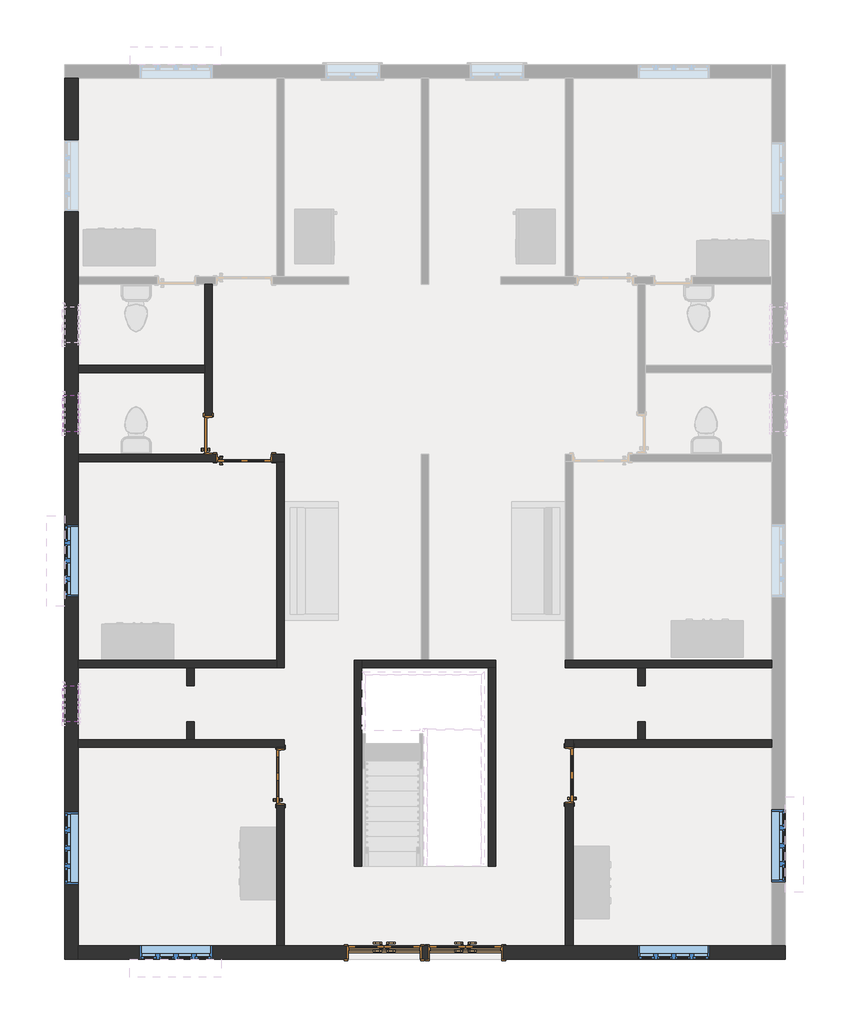
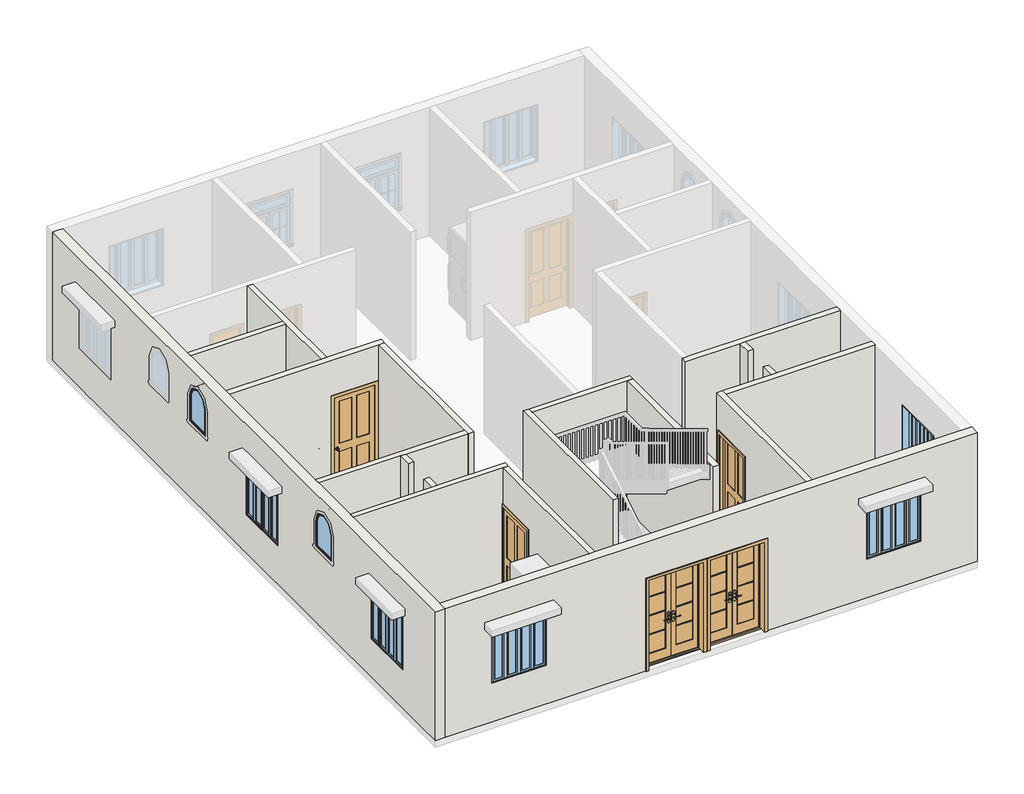
# One storey, part 1 of 4: 19 walls, 7 windows, 6 doors.
"""IFC4 building model written with IfcOpenShell, lengths in millimetres."""

from ifc_helpers import new_model, si_unit, frame, origin, origin_with_axes, place, context, project, spatial, polyline, circle_curve, outline, extrude, faceted_brep, transform, mapped, element, save
from ifc_brep_helpers import plane_surface, revolved_surface, advanced_brep
from components import door_exterior_double_full_glass_wood_clad_exterior_door_4_x_3788f36b, door_a823658d, door_68a706ac, door_3f5f64ee, window_casement_multi_sash_horizontal_main_windows_4_x_7_0e27d311, window_casement_multi_sash_horizontal_main_windows_4_x_7_c0e1ebbb, window_2fd4accf

model = new_model("IFC4")

# Units and contexts
model_context = context("Model", 3, world=origin())
ifc_project = project(units=[si_unit("LENGTHUNIT", "METRE", prefix="MILLI")], contexts=[model_context])

# Site, building, storey
site = spatial("IfcSite", under=ifc_project)
building = spatial("IfcBuilding", under=site)
storey = spatial("IfcBuildingStorey", under=building, Elevation=0.0)

# Doors
placement = place(None, origin())
door_exterior_double_full_glass_wood_clad_exterior_door_4_x_shape = door_exterior_double_full_glass_wood_clad_exterior_door_4_x_3788f36b(model_context)
element("IfcDoor", 1, ObjectType="Door-Exterior-Double-Full Glass-Wood_Clad : EXTERIOR DOOR 4' X 7'", at=placement, inside=storey, context=model_context, shape_type="MappedRepresentation", body=[
    mapped(door_exterior_double_full_glass_wood_clad_exterior_door_4_x_shape, transform((-10224.7771954, -6414.7977897, 0.0), x_axis=(1.0, 0.0, 0.0), y_axis=(0.0, 1.0, 0.0), z_axis=(0.0, 0.0, 1.0))),
])
element("IfcDoor", 2, ObjectType="Door-Exterior-Double-Full Glass-Wood_Clad : EXTERIOR DOOR 4' X 7'", at=placement, inside=storey, context=model_context, shape_type="MappedRepresentation", body=[
    mapped(door_exterior_double_full_glass_wood_clad_exterior_door_4_x_shape, transform((-8853.1771954, -6414.7977897, 0.0), x_axis=(1.0, 0.0, 0.0), y_axis=(0.0, 1.0, 0.0), z_axis=(0.0, 0.0, 1.0))),
])
door_shape = door_a823658d(model_context)
element("IfcDoor", 3, ObjectType="Door-Interior-Single-4_Panel-Wood : 36\" x 84\"", at=placement, inside=storey, context=model_context, shape_type="MappedRepresentation", body=[
    mapped(door_shape, transform((-7097.4021954, -3420.7727897, 0.0), x_axis=(0.0, 1.0, 0.0), y_axis=(-1.0, 0.0, 0.0), z_axis=(0.0, 0.0, 1.0))),
])
element("IfcDoor", 4, ObjectType="Door-Interior-Single-4_Panel-Wood : 36\" x 84\"", at=placement, inside=storey, context=model_context, shape_type="MappedRepresentation", body=[
    mapped(door_shape, transform((-12586.9771954, 1935.9816069, 0.0), x_axis=(1.0, 0.0, 0.0), y_axis=(0.0, 1.0, 0.0), z_axis=(0.0, 0.0, 1.0))),
])
door_2_shape = door_68a706ac(model_context)
element("IfcDoor", 5, ObjectType="Door-Interior-Single-4_Panel-Wood : 36\" x 84\"", at=placement, inside=storey, context=model_context, shape_type="MappedRepresentation", body=[
    mapped(door_2_shape, transform((-11980.5521954, -3446.1727897, 0.0), x_axis=(0.0, 1.0, 0.0), y_axis=(-1.0, 0.0, 0.0), z_axis=(0.0, 0.0, 1.0))),
])
door_3_shape = door_3f5f64ee(model_context)
element("IfcDoor", 6, ObjectType="Door-Interior-Single-Flush_Panel-Wood : 24\" x 84\"", at=placement, inside=storey, context=model_context, shape_type="MappedRepresentation", body=[
    mapped(door_3_shape, transform((-13199.7521954, 2320.1566069, 0.0), x_axis=(0.0, 1.0, 0.0), y_axis=(-1.0, 0.0, 0.0), z_axis=(0.0, 0.0, 1.0))),
])

# Walls
element("IfcWall", 7, ObjectType="INNER WALL 5\"", at=placement, inside=storey, context=model_context, shape_type="SweptSolid", body=[
    extrude(outline(polyline([(-13260.0771954, 3373.7272103), (-15395.2646954, 3373.7272103), (-15395.2646954, 3500.7272103), (-13260.0771954, 3500.7272103), (-13260.0771954, 3373.7272103)])), origin_with_axes(), (0.0, 0.0, 1.0), 3048.0),
])
element("IfcWall", 8, ObjectType="INNER WALL 5\"", at=placement, inside=storey, context=model_context, shape_type="Brep", body=[
    faceted_brep([(-13260.0771954, 4872.3272103, 3048.0), (-13260.0771954, 4872.3272103, 0.0), (-13260.0771954, 3500.7272103, 0.0), (-13260.0771954, 3373.7272103, 0.0), (-13260.0771954, 2650.3566069, 0.0), (-13260.0771954, 2650.3566069, 2159.0), (-13260.0771954, 2002.6566069, 2159.0), (-13260.0771954, 2002.6566069, 3048.0), (-13260.0771954, 3373.7272103, 3048.0), (-13260.0771954, 3500.7272103, 3048.0), (-13133.0771954, 4872.3272103, 0.0), (-13133.0771954, 4872.3272103, 3048.0), (-13133.0771954, 2002.6566069, 3048.0), (-13133.0771954, 2002.6566069, 2159.0), (-13133.0771954, 2650.3566069, 2159.0), (-13133.0771954, 2650.3566069, 0.0)], [[[0, 1, 2, 3, 4, 5, 6, 7, 8, 9]], [[10, 11, 12, 13, 14, 15]], [[1, 10, 15, 4, 3, 2]], [[1, 0, 11, 10]], [[12, 7, 6, 13]], [[14, 5, 4, 15]], [[5, 14, 13, 6]], [[0, 9, 8, 7, 12, 11]]]),
])
element("IfcWall", 9, ObjectType="INNER WALL 5\"", at=placement, inside=storey, context=model_context, shape_type="Brep", body=[
    faceted_brep([(-15395.2646954, 1875.6566069, 3048.0), (-15395.2646954, 1875.6566069, 0.0), (-13069.5771954, 1875.6566069, 0.0), (-13069.5771954, 1875.6566069, 2159.0), (-12104.3771954, 1875.6566069, 2159.0), (-12104.3771954, 1875.6566069, 0.0), (-12040.8771954, 1875.6566069, 0.0), (-11913.8771954, 1875.6566069, 0.0), (-11913.8771954, 1875.6566069, 3048.0), (-12040.8771954, 1875.6566069, 3048.0), (-15395.2646954, 2002.6566069, 0.0), (-15395.2646954, 2002.6566069, 3048.0), (-13260.0771954, 2002.6566069, 3048.0), (-13133.0771954, 2002.6566069, 3048.0), (-11913.8771954, 2002.6566069, 3048.0), (-11913.8771954, 2002.6566069, 0.0), (-12104.3771954, 2002.6566069, 0.0), (-12104.3771954, 2002.6566069, 2159.0), (-13069.5771954, 2002.6566069, 2159.0), (-13069.5771954, 2002.6566069, 0.0), (-13133.0771954, 2002.6566069, 0.0), (-13133.0771954, 2002.6566069, 2159.0), (-13260.0771954, 2002.6566069, 2159.0), (-13260.0771954, 2002.6566069, 0.0), (-13260.0771954, 1989.9566069, 0.0), (-13133.0771954, 1989.9566069, 0.0), (-13133.0771954, 1989.9566069, 2159.0), (-13260.0771954, 1989.9566069, 2159.0)], [[[0, 1, 2, 3, 4, 5, 6, 7, 8, 9]], [[10, 11, 12, 13, 14, 15, 16, 17, 18, 19, 20, 21, 22, 23]], [[1, 10, 23, 24, 25, 20, 19, 2]], [[15, 7, 6, 5, 16]], [[1, 0, 11, 10]], [[8, 7, 15, 14]], [[4, 17, 16, 5]], [[17, 4, 3, 18]], [[18, 3, 2, 19]], [[25, 26, 21, 20]], [[27, 24, 23, 22]], [[26, 27, 22, 21]], [[26, 25, 24, 27]], [[0, 9, 8, 14, 13, 12, 11]]]),
])
element("IfcWall", 10, ObjectType="INNER WALL 5\"", at=placement, inside=storey, context=model_context, shape_type="Brep", body=[
    faceted_brep([(-12040.8771954, 1875.6566069, 0.0), (-12040.8771954, -1477.6727897, 0.0), (-12040.8771954, -1604.6727897, 0.0), (-12040.8771954, -1604.6727897, 3048.0), (-12040.8771954, -1477.6727897, 3048.0), (-12040.8771954, 1875.6566069, 3048.0), (-11913.8771954, 1875.6566069, 0.0), (-11913.8771954, 1875.6566069, 3048.0), (-11913.8771954, -1604.6727897, 3048.0), (-11913.8771954, -1604.6727897, 0.0)], [[[0, 1, 2, 3, 4, 5]], [[6, 7, 8, 9]], [[2, 1, 0, 6, 9]], [[0, 5, 7, 6]], [[3, 2, 9, 8]], [[5, 4, 3, 8, 7]]]),
])
element("IfcWall", 11, ObjectType="INNER WALL 5\"", at=placement, inside=storey, context=model_context, shape_type="Brep", body=[
    faceted_brep([(-12040.8771954, -1477.6727897, 0.0), (-15395.2646954, -1477.6727897, 0.0), (-15395.2646954, -1477.6727897, 3048.0), (-12040.8771954, -1477.6727897, 3048.0), (-12040.8771954, -1604.6727897, 0.0), (-12040.8771954, -1604.6727897, 3048.0), (-13437.8771954, -1604.6727897, 3048.0), (-13564.8771954, -1604.6727897, 3048.0), (-15395.2646954, -1604.6727897, 3048.0), (-15395.2646954, -1604.6727897, 0.0), (-13564.8771954, -1604.6727897, 0.0), (-13437.8771954, -1604.6727897, 0.0)], [[[0, 1, 2, 3]], [[4, 5, 6, 7, 8, 9, 10, 11]], [[1, 0, 4, 11, 10, 9]], [[0, 3, 5, 4]], [[2, 1, 9, 8]], [[3, 2, 8, 7, 6, 5]]]),
])
element("IfcWall", 12, ObjectType="INNER WALL 5\"", at=placement, inside=storey, context=model_context, shape_type="Brep", body=[
    faceted_brep([(-15395.2646954, -2950.8727897, 0.0), (-12040.8771954, -2950.8727897, 0.0), (-11913.8771954, -2950.8727897, 0.0), (-11913.8771954, -2950.8727897, 3048.0), (-12040.8771954, -2950.8727897, 3048.0), (-15395.2646954, -2950.8727897, 3048.0), (-15395.2646954, -2823.8727897, 0.0), (-15395.2646954, -2823.8727897, 3048.0), (-13564.8771954, -2823.8727897, 3048.0), (-13437.8771954, -2823.8727897, 3048.0), (-11913.8771954, -2823.8727897, 3048.0), (-11913.8771954, -2823.8727897, 0.0), (-13437.8771954, -2823.8727897, 0.0), (-13564.8771954, -2823.8727897, 0.0)], [[[0, 1, 2, 3, 4, 5]], [[6, 7, 8, 9, 10, 11, 12, 13]], [[2, 1, 0, 6, 13, 12, 11]], [[0, 5, 7, 6]], [[3, 2, 11, 10]], [[5, 4, 3, 10, 9, 8, 7]]]),
])
element("IfcWall", 13, ObjectType="INNER WALL 5\"", at=placement, inside=storey, context=model_context, shape_type="SweptSolid", body=[
    extrude(outline(polyline([(-2950.8727897, 3048.0), (-2950.8727897, 0.0), (-2963.5727897, 0.0), (-2963.5727897, 2159.0), (-3928.7727897, 2159.0), (-3928.7727897, 0.0), (-6303.6727897, 0.0), (-6303.6727897, 3048.0), (-2950.8727897, 3048.0)])), frame((-12040.8771954, 0.0, 0.0), z_axis=(1.0, 0.0, 0.0), x_axis=(0.0, 1.0, 0.0)), (0.0, 0.0, 1.0), 127.0),
])
element("IfcWall", 14, ObjectType="INNER WALL 5\"", at=placement, inside=storey, context=model_context, shape_type="Brep", body=[
    faceted_brep([(-7037.0771954, -6303.6727897, 3048.0), (-7037.0771954, -6303.6727897, 0.0), (-7037.0771954, -3903.3727897, 0.0), (-7037.0771954, -3903.3727897, 2159.0), (-7037.0771954, -2938.1727897, 2159.0), (-7037.0771954, -2938.1727897, 0.0), (-7037.0771954, -2823.8727897, 0.0), (-7037.0771954, -2823.8727897, 3048.0), (-7037.0771954, -2950.8727897, 3048.0), (-7164.0771954, -6303.6727897, 0.0), (-7164.0771954, -6303.6727897, 3048.0), (-7164.0771954, -2823.8727897, 3048.0), (-7164.0771954, -2823.8727897, 0.0), (-7164.0771954, -2938.1727897, 0.0), (-7164.0771954, -2938.1727897, 2159.0), (-7164.0771954, -3903.3727897, 2159.0), (-7164.0771954, -3903.3727897, 0.0)], [[[0, 1, 2, 3, 4, 5, 6, 7, 8]], [[9, 10, 11, 12, 13, 14, 15, 16]], [[1, 9, 16, 2]], [[12, 6, 5, 13]], [[1, 0, 10, 9]], [[7, 6, 12, 11]], [[4, 14, 13, 5]], [[14, 4, 3, 15]], [[15, 3, 2, 16]], [[0, 8, 7, 11, 10]]]),
])
element("IfcWall", 15, ObjectType="INNER WALL 5\"", at=placement, inside=storey, context=model_context, shape_type="Brep", body=[
    faceted_brep([(-3684.2771954, -2823.8727897, 0.0), (-5817.8771954, -2823.8727897, 0.0), (-5944.8771954, -2823.8727897, 0.0), (-7037.0771954, -2823.8727897, 0.0), (-7037.0771954, -2823.8727897, 3048.0), (-5944.8771954, -2823.8727897, 3048.0), (-5817.8771954, -2823.8727897, 3048.0), (-3684.2771954, -2823.8727897, 3048.0), (-3684.2771954, -2950.8727897, 0.0), (-3684.2771954, -2950.8727897, 3048.0), (-7037.0771954, -2950.8727897, 3048.0), (-7037.0771954, -2950.8727897, 0.0)], [[[0, 1, 2, 3, 4, 5, 6, 7]], [[8, 9, 10, 11]], [[3, 2, 1, 0, 8, 11]], [[4, 3, 11, 10]], [[0, 7, 9, 8]], [[7, 6, 5, 4, 10, 9]]]),
])
element("IfcWall", 16, ObjectType="INNER WALL 5\"", at=placement, inside=storey, context=model_context, shape_type="Brep", body=[
    faceted_brep([(-3684.2771954, -1477.6727897, 0.0), (-7037.0771954, -1477.6727897, 0.0), (-7164.0771954, -1477.6727897, 0.0), (-7164.0771954, -1477.6727897, 3048.0), (-7037.0771954, -1477.6727897, 3048.0), (-3684.2771954, -1477.6727897, 3048.0), (-3684.2771954, -1604.6727897, 0.0), (-3684.2771954, -1604.6727897, 3048.0), (-5817.8771954, -1604.6727897, 3048.0), (-5944.8771954, -1604.6727897, 3048.0), (-7164.0771954, -1604.6727897, 3048.0), (-7164.0771954, -1604.6727897, 0.0), (-5944.8771954, -1604.6727897, 0.0), (-5817.8771954, -1604.6727897, 0.0)], [[[0, 1, 2, 3, 4, 5]], [[6, 7, 8, 9, 10, 11, 12, 13]], [[2, 1, 0, 6, 13, 12, 11]], [[0, 5, 7, 6]], [[3, 2, 11, 10]], [[5, 4, 3, 10, 9, 8, 7]]]),
])
element("IfcWall", 17, ObjectType="INNER WALL 5\"", at=placement, inside=storey, context=model_context, shape_type="SweptSolid", body=[
    extrude(outline(polyline([(-13564.8771954, -1909.4727897), (-13564.8771954, -1604.6727897), (-13437.8771954, -1604.6727897), (-13437.8771954, -1909.4727897), (-13564.8771954, -1909.4727897)])), origin_with_axes(), (0.0, 0.0, 1.0), 3048.0),
])
element("IfcWall", 18, ObjectType="INNER WALL 5\"", at=placement, inside=storey, context=model_context, shape_type="SweptSolid", body=[
    extrude(outline(polyline([(-13437.8771954, -2519.0727897), (-13437.8771954, -2823.8727897), (-13564.8771954, -2823.8727897), (-13564.8771954, -2519.0727897), (-13437.8771954, -2519.0727897)])), origin_with_axes(), (0.0, 0.0, 1.0), 3048.0),
])
element("IfcWall", 19, ObjectType="INNER WALL 5\"", at=placement, inside=storey, context=model_context, shape_type="SweptSolid", body=[
    extrude(outline(polyline([(-5817.8771954, -2519.0727897), (-5817.8771954, -2823.8727897), (-5944.8771954, -2823.8727897), (-5944.8771954, -2519.0727897), (-5817.8771954, -2519.0727897)])), origin_with_axes(), (0.0, 0.0, 1.0), 3048.0),
])
element("IfcWall", 20, ObjectType="INNER WALL 5\"", at=placement, inside=storey, context=model_context, shape_type="SweptSolid", body=[
    extrude(outline(polyline([(-5944.8771954, -1909.4727897), (-5944.8771954, -1604.6727897), (-5817.8771954, -1604.6727897), (-5817.8771954, -1909.4727897), (-5944.8771954, -1909.4727897)])), origin_with_axes(), (0.0, 0.0, 1.0), 3048.0),
])
element("IfcWall", 21, ObjectType="INNER WALL 5\"", at=placement, inside=storey, context=model_context, shape_type="Brep", body=[
    faceted_brep([(-10605.7771954, -4957.4727897, 0.0), (-10605.7771954, -1604.6727897, 0.0), (-10605.7771954, -1477.6727897, 0.0), (-10605.7771954, -1477.6727897, 3048.0), (-10605.7771954, -1604.6727897, 3048.0), (-10605.7771954, -4957.4727897, 3048.0), (-10732.7771954, -4957.4727897, 0.0), (-10732.7771954, -4957.4727897, 3048.0), (-10732.7771954, -1477.6727897, 3048.0), (-10732.7771954, -1477.6727897, 0.0)], [[[0, 1, 2, 3, 4, 5]], [[6, 7, 8, 9]], [[2, 1, 0, 6, 9]], [[0, 5, 7, 6]], [[3, 2, 9, 8]], [[5, 4, 3, 8, 7]]]),
])
element("IfcWall", 22, ObjectType="INNER WALL 5\"", at=placement, inside=storey, context=model_context, shape_type="Brep", body=[
    faceted_brep([(-10605.7771954, -1604.6727897, 0.0), (-8472.1771954, -1604.6727897, 0.0), (-8345.1771954, -1604.6727897, 0.0), (-8345.1771954, -1604.6727897, 3048.0), (-8472.1771954, -1604.6727897, 3048.0), (-10605.7771954, -1604.6727897, 3048.0), (-10605.7771954, -1477.6727897, 0.0), (-10605.7771954, -1477.6727897, 3048.0), (-9602.4771954, -1477.6727897, 3048.0), (-9475.4771954, -1477.6727897, 3048.0), (-8345.1771954, -1477.6727897, 3048.0), (-8345.1771954, -1477.6727897, 0.0), (-9475.4771954, -1477.6727897, 0.0), (-9602.4771954, -1477.6727897, 0.0)], [[[0, 1, 2, 3, 4, 5]], [[6, 7, 8, 9, 10, 11, 12, 13]], [[2, 1, 0, 6, 13, 12, 11]], [[0, 5, 7, 6]], [[3, 2, 11, 10]], [[5, 4, 3, 10, 9, 8, 7]]]),
])
element("IfcWall", 23, ObjectType="INNER WALL 5\"", at=placement, inside=storey, context=model_context, shape_type="SweptSolid", body=[
    extrude(outline(polyline([(-8472.1771954, -4957.4727897), (-8472.1771954, -1604.6727897), (-8345.1771954, -1604.6727897), (-8345.1771954, -4957.4727897), (-8472.1771954, -4957.4727897)])), origin_with_axes(), (0.0, 0.0, 1.0), 3048.0),
])
element("IfcWall", 24, ObjectType="OUTER WALL 9\"", at=placement, inside=storey, context=model_context, shape_type="AdvancedBrep", body=[
    advanced_brep(
    [(-15395.2646954, -6532.2727897, 0.0), (-15395.2646954, -6303.6727897, 0.0), (-15395.2646954, -2950.8727897, 0.0), (-15395.2646954, -2823.8727897, 0.0), (-15395.2646954, -1604.6727897, 0.0), (-15395.2646954, -1477.6727897, 0.0), (-15395.2646954, 1875.6566069, 0.0), (-15395.2646954, 2002.6566069, 0.0), (-15395.2646954, 3373.7272103, 0.0), (-15395.2646954, 3500.7272103, 0.0), (-15395.2646954, 4872.3272103, 0.0), (-15395.2646954, 4999.3272103, 0.0), (-15395.2646954, 8352.1272103, 0.0), (-15395.2646954, 8352.1272103, 3048.0), (-15395.2646954, 4999.3272103, 3048.0), (-15395.2646954, 4872.3272103, 3048.0), (-15395.2646954, 3500.7272103, 3048.0), (-15395.2646954, 3373.7272103, 3048.0), (-15395.2646954, 2002.6566069, 3048.0), (-15395.2646954, 1875.6566069, 3048.0), (-15395.2646954, -1477.6727897, 3048.0), (-15395.2646954, -1604.6727897, 3048.0), (-15395.2646954, -2823.8727897, 3048.0), (-15395.2646954, -2950.8727897, 3048.0), (-15395.2646954, -6303.6727897, 3048.0), (-15395.2646954, -6532.2727897, 3048.0), (-15395.2646954, -4043.0727897, 2260.6), (-15395.2646954, -4043.0727897, 914.4), (-15395.2646954, -5262.2727897, 914.4), (-15395.2646954, -5262.2727897, 2260.6), (-15395.2646954, 808.5919086, 2260.6), (-15395.2646954, 808.5919086, 914.4), (-15395.2646954, -410.6080914, 914.4), (-15395.2646954, -410.6080914, 2260.6), (-15395.2646954, 7310.7272103, 2260.6), (-15395.2646954, 7310.7272103, 914.4), (-15395.2646954, 6091.5272103, 914.4), (-15395.2646954, 6091.5272103, 2260.6), (-15395.2646954, -2519.0727897, 1828.8), (-15395.2646954, -2519.0727897, 2438.4), (-15395.2646954, -1909.4727897, 2438.4), (-15395.2646954, -1909.4727897, 1828.8), (-15395.2646954, 2383.3919086, 1828.8), (-15395.2646954, 2383.3919086, 2438.4), (-15395.2646954, 2992.9919086, 2438.4), (-15395.2646954, 2992.9919086, 1828.8), (-15395.2646954, 3881.7272103, 1828.8), (-15395.2646954, 3881.7272103, 2438.4), (-15395.2646954, 4491.3272103, 2438.4), (-15395.2646954, 4491.3272103, 1828.8), (-15623.8646954, -6532.2727897, 0.0), (-15623.8646954, -6532.2727897, 3048.0), (-15623.8646954, 8352.1272103, 3048.0), (-15623.8646954, 8352.1272103, 0.0), (-15623.8646954, -4043.0727897, 2260.6), (-15623.8646954, -5262.2727897, 2260.6), (-15623.8646954, -5262.2727897, 914.4), (-15623.8646954, -4043.0727897, 914.4), (-15623.8646954, 808.5919086, 2260.6), (-15623.8646954, -410.6080914, 2260.6), (-15623.8646954, -410.6080914, 914.4), (-15623.8646954, 808.5919086, 914.4), (-15623.8646954, 7310.7272103, 2260.6), (-15623.8646954, 6091.5272103, 2260.6), (-15623.8646954, 6091.5272103, 914.4), (-15623.8646954, 7310.7272103, 914.4), (-15623.8646954, -2519.0727897, 1828.8), (-15623.8646954, -1909.4727897, 1828.8), (-15623.8646954, -1909.4727897, 2438.4), (-15623.8646954, -2519.0727897, 2438.4), (-15623.8646954, 2383.3919086, 1828.8), (-15623.8646954, 2992.9919086, 1828.8), (-15623.8646954, 2992.9919086, 2438.4), (-15623.8646954, 2383.3919086, 2438.4), (-15623.8646954, 3881.7272103, 1828.8), (-15623.8646954, 4491.3272103, 1828.8), (-15623.8646954, 4491.3272103, 2438.4), (-15623.8646954, 3881.7272103, 2438.4)],
    [
        (0, 1),
        (1, 2),
        (2, 3),
        (3, 4),
        (4, 5),
        (5, 6),
        (6, 7),
        (7, 8),
        (8, 9),
        (9, 10),
        (10, 11),
        (11, 12),
        (12, 13),
        (13, 14),
        (14, 15),
        (15, 16),
        (16, 17),
        (17, 18),
        (18, 19),
        (19, 20),
        (20, 21),
        (21, 22),
        (22, 23),
        (23, 24),
        (24, 25),
        (25, 0),
        (26, 27),
        (27, 28),
        (28, 29),
        (29, 26),
        (30, 31),
        (31, 32),
        (32, 33),
        (33, 30),
        (34, 35),
        (35, 36),
        (36, 37),
        (37, 34),
        (38, 39),
        (39, 40, circle_curve(frame((-15395.2646954, -2214.2727897, 2438.4), z_axis=(-1.0, 0.0, 0.0), x_axis=(0.0, 1.0, 0.0)), 304.8)),
        (40, 41),
        (41, 38),
        (42, 43),
        (43, 44, circle_curve(frame((-15395.2646954, 2688.1919086, 2438.4), z_axis=(-1.0, 0.0, 0.0), x_axis=(0.0, 1.0, 0.0)), 304.8)),
        (44, 45),
        (45, 42),
        (46, 47),
        (47, 48, circle_curve(frame((-15395.2646954, 4186.5272103, 2438.4), z_axis=(-1.0, 0.0, 0.0), x_axis=(0.0, 1.0, 0.0)), 304.8)),
        (48, 49),
        (49, 46),
        (50, 51),
        (51, 52),
        (52, 53),
        (53, 50),
        (54, 55),
        (55, 56),
        (56, 57),
        (57, 54),
        (58, 59),
        (59, 60),
        (60, 61),
        (61, 58),
        (62, 63),
        (63, 64),
        (64, 65),
        (65, 62),
        (66, 67),
        (67, 68),
        (68, 69, circle_curve(frame((-15623.8646954, -2214.2727897, 2438.4), z_axis=(1.0, 0.0, 0.0), x_axis=(0.0, 1.0, 0.0)), 304.8)),
        (69, 66),
        (70, 71),
        (71, 72),
        (72, 73, circle_curve(frame((-15623.8646954, 2688.1919086, 2438.4), z_axis=(1.0, 0.0, 0.0), x_axis=(0.0, 1.0, 0.0)), 304.8)),
        (73, 70),
        (74, 75),
        (75, 76),
        (76, 77, circle_curve(frame((-15623.8646954, 4186.5272103, 2438.4), z_axis=(1.0, 0.0, 0.0), x_axis=(0.0, 1.0, 0.0)), 304.8)),
        (77, 74),
        (0, 50),
        (53, 12),
        (25, 51),
        (52, 13),
        (26, 54),
        (57, 27),
        (56, 28),
        (55, 29),
        (30, 58),
        (61, 31),
        (60, 32),
        (59, 33),
        (34, 62),
        (65, 35),
        (64, 36),
        (63, 37),
        (66, 38),
        (41, 67),
        (40, 68),
        (39, 69),
        (70, 42),
        (45, 71),
        (44, 72),
        (43, 73),
        (74, 46),
        (49, 75),
        (48, 76),
        (47, 77),
    ],
    [
        plane_surface(frame((-15395.2646954, 7399.6272103, 0.0), z_axis=(1.0, 0.0, 0.0), x_axis=(0.0, 1.0, 0.0))),
        plane_surface(frame((-15623.8646954, 7399.6272103, 0.0), z_axis=(-1.0, 0.0, 0.0), x_axis=(0.0, -1.0, 0.0))),
        plane_surface(frame((-15395.2646954, -6417.9727897, 0.0), z_axis=(0.0, 0.0, -1.0), x_axis=(-1.0, 0.0, 0.0))),
        plane_surface(frame((-3569.9771954, -6532.2727897, 0.0), z_axis=(0.0, -1.0, 0.0), x_axis=(1.0, 0.0, 0.0))),
        plane_surface(frame((-15509.5646954, 8352.1272103, 0.0), z_axis=(0.0, 1.0, 0.0), x_axis=(1.0, 0.0, 0.0))),
        plane_surface(frame((-15395.2646954, -4043.0727897, 2260.6), z_axis=(0.0, -1.0, 0.0), x_axis=(-1.0, 0.0, 0.0))),
        plane_surface(frame((-15395.2646954, -4043.0727897, 914.4), z_axis=(0.0, 0.0, 1.0), x_axis=(-1.0, 0.0, 0.0))),
        plane_surface(frame((-15395.2646954, -5262.2727897, 914.4), z_axis=(0.0, 1.0, 0.0), x_axis=(-1.0, 0.0, 0.0))),
        plane_surface(frame((-15395.2646954, -5262.2727897, 2260.6), z_axis=(0.0, 0.0, -1.0), x_axis=(-1.0, 0.0, 0.0))),
        plane_surface(frame((-15395.2646954, 808.5919086, 2260.6), z_axis=(0.0, -1.0, 0.0), x_axis=(-1.0, 0.0, 0.0))),
        plane_surface(frame((-15395.2646954, 808.5919086, 914.4), z_axis=(0.0, 0.0, 1.0), x_axis=(-1.0, 0.0, 0.0))),
        plane_surface(frame((-15395.2646954, -410.6080914, 914.4), z_axis=(0.0, 1.0, 0.0), x_axis=(-1.0, 0.0, 0.0))),
        plane_surface(frame((-15395.2646954, -410.6080914, 2260.6), z_axis=(0.0, 0.0, -1.0), x_axis=(-1.0, 0.0, 0.0))),
        plane_surface(frame((-15395.2646954, 7310.7272103, 2260.6), z_axis=(0.0, -1.0, 0.0), x_axis=(-1.0, 0.0, 0.0))),
        plane_surface(frame((-15395.2646954, 7310.7272103, 914.4), z_axis=(0.0, 0.0, 1.0), x_axis=(-1.0, 0.0, 0.0))),
        plane_surface(frame((-15395.2646954, 6091.5272103, 914.4), z_axis=(0.0, 1.0, 0.0), x_axis=(-1.0, 0.0, 0.0))),
        plane_surface(frame((-15395.2646954, 6091.5272103, 2260.6), z_axis=(0.0, 0.0, -1.0), x_axis=(-1.0, 0.0, 0.0))),
        plane_surface(frame((-15623.8646954, -2519.0727897, 1828.8), z_axis=(0.0, 0.0, 1.0), x_axis=(1.0, 0.0, 0.0))),
        plane_surface(frame((-15623.8646954, -1909.4727897, 1828.8), z_axis=(0.0, -1.0, 0.0), x_axis=(1.0, 0.0, 0.0))),
        revolved_surface(polyline([(-15395.2646954, -1909.4727897, 2438.4), (-15623.8646954, -1909.4727897, 2438.4)]), (-15395.2646954, -2214.2727897, 2438.4), (1.0, 0.0, 0.0)),
        plane_surface(frame((-15623.8646954, -2519.0727897, 2438.4), z_axis=(0.0, 1.0, 0.0), x_axis=(1.0, 0.0, 0.0))),
        plane_surface(frame((-15623.8646954, 2383.3919086, 1828.8), z_axis=(0.0, 0.0, 1.0), x_axis=(1.0, 0.0, 0.0))),
        plane_surface(frame((-15623.8646954, 2992.9919086, 1828.8), z_axis=(0.0, -1.0, 0.0), x_axis=(1.0, 0.0, 0.0))),
        revolved_surface(polyline([(-15395.2646954, 2992.9919086, 2438.4), (-15623.8646954, 2992.9919086, 2438.4)]), (-15395.2646954, 2688.1919086, 2438.4), (1.0, 0.0, 0.0)),
        plane_surface(frame((-15623.8646954, 2383.3919086, 2438.4), z_axis=(0.0, 1.0, 0.0), x_axis=(1.0, 0.0, 0.0))),
        plane_surface(frame((-15623.8646954, 3881.7272103, 1828.8), z_axis=(0.0, 0.0, 1.0), x_axis=(1.0, 0.0, 0.0))),
        plane_surface(frame((-15623.8646954, 4491.3272103, 1828.8), z_axis=(0.0, -1.0, 0.0), x_axis=(1.0, 0.0, 0.0))),
        revolved_surface(polyline([(-15395.2646954, 4491.3272103, 2438.4), (-15623.8646954, 4491.3272103, 2438.4)]), (-15395.2646954, 4186.5272103, 2438.4), (1.0, 0.0, 0.0)),
        plane_surface(frame((-15623.8646954, 3881.7272103, 2438.4), z_axis=(0.0, 1.0, 0.0), x_axis=(1.0, 0.0, 0.0))),
        plane_surface(frame((-15623.8646954, 8580.7272103, 3048.0), z_axis=(0.0, 0.0, 1.0), x_axis=(1.0, 0.0, 0.0))),
    ],
    [
        (0, [[1, 2, 3, 4, 5, 6, 7, 8, 9, 10, 11, 12, 13, 14, 15, 16, 17, 18, 19, 20, 21, 22, 23, 24, 25, 26], [27, 28, 29, 30], [31, 32, 33, 34], [35, 36, 37, 38], [39, 40, 41, 42], [43, 44, 45, 46], [47, 48, 49, 50]]),
        (1, [[51, 52, 53, 54], [55, 56, 57, 58], [59, 60, 61, 62], [63, 64, 65, 66], [67, 68, 69, 70], [71, 72, 73, 74], [75, 76, 77, 78]]),
        (2, [[-12, -11, -10, -9, -8, -7, -6, -5, -4, -3, -2, -1, 79, -54, 80]]),
        (3, [[-26, 81, -51, -79]]),
        (4, [[-13, -80, -53, 82]]),
        (5, [[-27, 83, -58, 84]]),
        (6, [[-28, -84, -57, 85]]),
        (7, [[-29, -85, -56, 86]]),
        (8, [[-30, -86, -55, -83]]),
        (9, [[-31, 87, -62, 88]]),
        (10, [[-32, -88, -61, 89]]),
        (11, [[-33, -89, -60, 90]]),
        (12, [[-34, -90, -59, -87]]),
        (13, [[-35, 91, -66, 92]]),
        (14, [[-36, -92, -65, 93]]),
        (15, [[-37, -93, -64, 94]]),
        (16, [[-38, -94, -63, -91]]),
        (17, [[-67, 95, -42, 96]]),
        (18, [[-68, -96, -41, 97]]),
        (19, [[-69, -97, -40, 98]]),
        (20, [[-70, -98, -39, -95]]),
        (21, [[-71, 99, -46, 100]]),
        (22, [[-72, -100, -45, 101]]),
        (23, [[-73, -101, -44, 102]]),
        (24, [[-74, -102, -43, -99]]),
        (25, [[-75, 103, -50, 104]]),
        (26, [[-76, -104, -49, 105]]),
        (27, [[-77, -105, -48, 106]]),
        (28, [[-78, -106, -47, -103]]),
        (29, [[-25, -24, -23, -22, -21, -20, -19, -18, -17, -16, -15, -14, -82, -52, -81]]),
    ],
),
])
element("IfcWall", 25, ObjectType="OUTER WALL 9\"", at=placement, inside=storey, context=model_context, shape_type="Brep", body=[
    faceted_brep([(-3455.6771954, -6303.6727897, 3048.0), (-3455.6771954, -6303.6727897, 0.0), (-3684.2771954, -6303.6727897, 0.0), (-7037.0771954, -6303.6727897, 0.0), (-7164.0771954, -6303.6727897, 0.0), (-8218.1771954, -6303.6727897, 0.0), (-8218.1771954, -6303.6727897, 2159.0), (-9488.1771954, -6303.6727897, 2159.0), (-9488.1771954, -6303.6727897, 0.0), (-9589.7771954, -6303.6727897, 0.0), (-9589.7771954, -6303.6727897, 2159.0), (-10859.7771954, -6303.6727897, 2159.0), (-10859.7771954, -6303.6727897, 0.0), (-11913.8771954, -6303.6727897, 0.0), (-12040.8771954, -6303.6727897, 0.0), (-15395.2646954, -6303.6727897, 0.0), (-15395.2646954, -6303.6727897, 3048.0), (-12040.8771954, -6303.6727897, 3048.0), (-11913.8771954, -6303.6727897, 3048.0), (-7164.0771954, -6303.6727897, 3048.0), (-7037.0771954, -6303.6727897, 3048.0), (-3684.2771954, -6303.6727897, 3048.0), (-14353.0709454, -6303.6727897, 2260.6), (-14353.0709454, -6303.6727897, 914.4), (-13133.8709454, -6303.6727897, 914.4), (-13133.8709454, -6303.6727897, 2260.6), (-5944.8771954, -6303.6727897, 2260.6), (-5944.8771954, -6303.6727897, 914.4), (-4725.6771954, -6303.6727897, 914.4), (-4725.6771954, -6303.6727897, 2260.6), (-3455.6771954, -6532.2727897, 0.0), (-3455.6771954, -6532.2727897, 3048.0), (-15395.2646954, -6532.2727897, 3048.0), (-15395.2646954, -6532.2727897, 0.0), (-10859.7771954, -6532.2727897, 0.0), (-10859.7771954, -6532.2727897, 2159.0), (-9589.7771954, -6532.2727897, 2159.0), (-9589.7771954, -6532.2727897, 0.0), (-9488.1771954, -6532.2727897, 0.0), (-9488.1771954, -6532.2727897, 2159.0), (-8218.1771954, -6532.2727897, 2159.0), (-8218.1771954, -6532.2727897, 0.0), (-14353.0709454, -6532.2727897, 2260.6), (-13133.8709454, -6532.2727897, 2260.6), (-13133.8709454, -6532.2727897, 914.4), (-14353.0709454, -6532.2727897, 914.4), (-5944.8771954, -6532.2727897, 2260.6), (-4725.6771954, -6532.2727897, 2260.6), (-4725.6771954, -6532.2727897, 914.4), (-5944.8771954, -6532.2727897, 914.4)], [[[0, 1, 2, 3, 4, 5, 6, 7, 8, 9, 10, 11, 12, 13, 14, 15, 16, 17, 18, 19, 20, 21], [22, 23, 24, 25], [26, 27, 28, 29]], [[30, 31, 32, 33, 34, 35, 36, 37, 38, 39, 40, 41], [42, 43, 44, 45], [46, 47, 48, 49]], [[1, 30, 41, 5, 4, 3, 2]], [[33, 15, 14, 13, 12, 34]], [[37, 9, 8, 38]], [[1, 0, 31, 30]], [[16, 15, 33, 32]], [[36, 10, 9, 37]], [[10, 36, 35, 11]], [[11, 35, 34, 12]], [[40, 6, 5, 41]], [[6, 40, 39, 7]], [[7, 39, 38, 8]], [[23, 22, 42, 45]], [[24, 23, 45, 44]], [[25, 24, 44, 43]], [[22, 25, 43, 42]], [[27, 26, 46, 49]], [[28, 27, 49, 48]], [[29, 28, 48, 47]], [[26, 29, 47, 46]], [[0, 21, 20, 19, 18, 17, 16, 32, 31]]]),
])

# Windows
window_casement_multi_sash_horizontal_main_windows_4_x_7_shape = window_casement_multi_sash_horizontal_main_windows_4_x_7_0e27d311(model_context)
element("IfcWindow", 26, ObjectType="Window-Casement-Multi-Sash-Horizontal : MAIN WINDOWS 4' X 7'", at=placement, inside=storey, context=model_context, shape_type="MappedRepresentation", body=[
    mapped(window_casement_multi_sash_horizontal_main_windows_4_x_7_shape, transform((-13743.4709454, -6417.9727897, 0.0), x_axis=(-1.0, 0.0, 0.0), y_axis=(0.0, -1.0, 0.0), z_axis=(0.0, 0.0, 1.0))),
])
element("IfcWindow", 27, ObjectType="Window-Casement-Multi-Sash-Horizontal : MAIN WINDOWS 4' X 7'", at=placement, inside=storey, context=model_context, shape_type="MappedRepresentation", body=[
    mapped(window_casement_multi_sash_horizontal_main_windows_4_x_7_shape, transform((-5335.2771954, -6417.9727897, 0.0), x_axis=(-1.0, 0.0, 0.0), y_axis=(0.0, -1.0, 0.0), z_axis=(0.0, 0.0, 1.0))),
])
element("IfcWindow", 28, ObjectType="Window-Casement-Multi-Sash-Horizontal : MAIN WINDOWS 4' X 7'", at=placement, inside=storey, context=model_context, shape_type="MappedRepresentation", body=[
    mapped(window_casement_multi_sash_horizontal_main_windows_4_x_7_shape, transform((-15509.5646954, -4652.6727897, 0.0), x_axis=(0.0, 1.0, 0.0), y_axis=(-1.0, 0.0, 0.0), z_axis=(0.0, 0.0, 1.0))),
])
element("IfcWindow", 29, ObjectType="Window-Casement-Multi-Sash-Horizontal : MAIN WINDOWS 4' X 7'", at=placement, inside=storey, context=model_context, shape_type="MappedRepresentation", body=[
    mapped(window_casement_multi_sash_horizontal_main_windows_4_x_7_shape, transform((-15509.5646954, 198.9919086, 0.0), x_axis=(0.0, 1.0, 0.0), y_axis=(-1.0, 0.0, 0.0), z_axis=(0.0, 0.0, 1.0))),
])
window_casement_multi_sash_horizontal_main_windows_4_x_7_2_shape = window_casement_multi_sash_horizontal_main_windows_4_x_7_c0e1ebbb(model_context)
element("IfcWindow", 30, ObjectType="Window-Casement-Multi-Sash-Horizontal : MAIN WINDOWS 4' X 7'", at=placement, inside=storey, context=model_context, shape_type="MappedRepresentation", body=[
    mapped(window_casement_multi_sash_horizontal_main_windows_4_x_7_2_shape, transform((-3569.9771954, -4614.5727897, 0.0), x_axis=(0.0, 1.0, 0.0), y_axis=(-1.0, 0.0, 0.0), z_axis=(0.0, 0.0, 1.0))),
])
window_shape = window_2fd4accf(model_context)
element("IfcWindow", 31, ObjectType="Window-Fixed-Round-Top : 24\" x 36\"", at=placement, inside=storey, context=model_context, shape_type="MappedRepresentation", body=[
    mapped(window_shape, transform((-15509.5646954, -2214.2727897, 914.4), x_axis=(0.0, 1.0, 0.0), y_axis=(-1.0, 0.0, 0.0), z_axis=(0.0, 0.0, 1.0))),
])
element("IfcWindow", 32, ObjectType="Window-Fixed-Round-Top : 24\" x 36\"", at=placement, inside=storey, context=model_context, shape_type="MappedRepresentation", body=[
    mapped(window_shape, transform((-15509.5646954, 2688.1919086, 914.4), x_axis=(0.0, 1.0, 0.0), y_axis=(-1.0, 0.0, 0.0), z_axis=(0.0, 0.0, 1.0))),
])

save(model, "model.ifc")

# Revit data of these elements
# Type "Door-Exterior-Double-Full Glass-Wood_Clad : EXTERIOR DOOR 4' X 7'"
#   Type Mark = "9"
#   Assembly Code = "B2030100"
#   Analytic Construction = "French door, wood frame with double glass"
#   Top Rail = 0' - 4 11/16"
#   Threshold Offset [instance default] = 0' - 0 1/2"
#   Thickness = 0' - 1 3/8"
#   Thermal Resistance (R) = 1.9158 (h·ft²·°F)/BTU
#   Swing Angle [instance default] = 90.00°
#   Stiles = 0' - 4 3/4"
#   Rough Width = 4' - 2"
#   Rough Height = 7' - 1"
#   Panel Width = 2' - 0"
#   Door Offset [instance default] = 0' - 0"
#   Height = 7' - 0"
#   Width = 4' - 0"
#   Heat Transfer Coefficient (U) = 0.5220 BTU/(h·ft²·°F)
#   Bottom Rail = 0' - 9 1/8"
#   Exterior Trim [instance default] = yes
#   Threshold [instance default] = yes
#   Show Grill [instance default] = yes
#   Function = 1
#   Trim Material = Cherry
#   Threshold Material = Cherry
#   Panel Material = Cherry
#   Glazing = Glass
#   Frame Material = Cherry
#   Door Handle Material = Aluminum
#   Visual Light Transmittance = 0
#   Solar Heat Gain Coefficient = 0
#   Wall Closure = (empty or 0)
#   Construction Type = (empty or 0)
# Type "Door-Interior-Single-4_Panel-Wood : 36\" x 84\""
#   Type Mark = "10"
#   Assembly Code = "C1020300"
#   Analytic Construction = "Wooden"
#   Top Rail = 0' - 4 11/16"
#   Thickness = 0' - 1 3/8"
#   Thermal Resistance (R) = 2.5876 (h·ft²·°F)/BTU
#   Swing Angle [instance default] = 90.00°
#   Stiles = 0' - 4 3/4"
#   Rough Width = 3' - 2"
#   Rough Height = 7' - 1"
#   Mullion = 0' - 4 1/2"
#   Lock Rail = 0' - 7 1/2"
#   Height = 7' - 0"
#   Width = 3' - 0"
#   Heat Transfer Coefficient (U) = 0.3865 BTU/(h·ft²·°F)
#   Bottom Rail = 0' - 9 1/8"
#   Trim Material = Cherry
#   Panel Material = Cherry
#   Frame Material = Cherry
#   Door Handle Material = Aluminum
#   Visual Light Transmittance = 0
#   Solar Heat Gain Coefficient = 0
#   Wall Closure = (empty or 0)
#   Function = (empty or 0)
# Type "Door-Interior-Single-Flush_Panel-Wood : 24\" x 84\""
#   Type Mark = "11"
#   Assembly Code = "C1020300"
#   Analytic Construction = "Wooden"
#   Thickness = 0' - 1 3/8"
#   Thermal Resistance (R) = 2.5876 (h·ft²·°F)/BTU
#   Swing Angle [instance default] = 90.00°
#   Rough Width = 2' - 2"
#   Rough Height = 7' - 1"
#   Height = 7' - 0"
#   Width = 2' - 0"
#   Heat Transfer Coefficient (U) = 0.3865 BTU/(h·ft²·°F)
#   Trim Material = Cherry
#   Panel Material = Cherry
#   Frame Material = Cherry
#   Door Handle Material = Aluminum
#   Visual Light Transmittance = 0
#   Solar Heat Gain Coefficient = 0
#   Wall Closure = (empty or 0)
#   Function = (empty or 0)
# Type "INNER WALL 5\""
#   Assembly Code = "B2010"
#   Layers, outside or top first: 0' - 5" "OUTER WALL PAINT" (function 1)
# Type "OUTER WALL 9\""
#   Assembly Code = "B2010"
#   Layers, outside or top first: 0' - 9" "OUTER WALL PAINT" (function 1)
# Type "Window-Casement-Multi-Sash-Horizontal : MAIN WINDOWS 4' X 7'"
#   Type Mark = "21"
#   Fire Rating = "0.5h"
#   Assembly Code = "B2020100"
#   Analytic Construction = "Double glazing - domestic"
#   Window Inset [instance default] = 0' - 0 5/8"
#   Wall Thickness [instance default] = 0' - 6"
#   Visual Light Transmittance = 0.81
#   Thermal Resistance (R) = 1.8146 (h·ft²·°F)/BTU
#   Solar Heat Gain Coefficient = 0.76
#   Rough Width = 4' - 0 1/2"
#   Rough Height = 4' - 5 1/2"
#   Open Window Width = 1' - 0"
#   Heat Transfer Coefficient (U) = 0.5511 BTU/(h·ft²·°F)
#   Height = 4' - 5"
#   Frame Gap 3 [instance default] = 0' - 1 83/128"
#   Frame Gap 2 [instance default] = 0' - 0 5/8"
#   Frame Gap 1 = 0' - 1 51/128"
#   Default Sill Height = 3' - 0"
#   Width = 4' - 0"
#   Frame Material = Metal - Aluminum
#   Glass Panel Material = Glass
#   Wall Closure = (empty or 0)
# Type "Window-Fixed-Round-Top : 24\" x 36\""
#   Type Mark = "31"
#   Fire Rating = "0.5h"
#   Assembly Code = "B2020100"
#   Analytic Construction = "Double glazing - domestic"
#   Window Inset [instance default] = 0' - 0"
#   Wall Thickness [instance default] = 0' - 6"
#   Visual Light Transmittance = 0.81
#   Thermal Resistance (R) = 1.8146 (h·ft²·°F)/BTU
#   Solar Heat Gain Coefficient = 0.76
#   Rough Width = 2' - 0 1/2"
#   Rough Height = 3' - 0 1/2"
#   Interior Wall Closure [instance default] = 0' - 2 1/4"
#   Height = 3' - 0"
#   Heat Transfer Coefficient (U) = 0.5511 BTU/(h·ft²·°F)
#   Frame Extension [instance default] = 0' - 0 1/4"
#   Exterior Wall Closure [instance default] = 0' - 1 1/4"
#   Extension Jamb [instance default] = 0' - 2 1/4"
#   Default Sill Height = 3' - 0"
#   Width = 2' - 0"
#   Interior Trim Visibility [instance default] = yes
#   Exterior Trim Visibility [instance default] = yes
#   Extension Jamb Visibility [instance default] = yes
#   Interior Trim Material = Wood - Stained
#   Interior Trim = Trim-Window-Interior-Flat-Arch-Top-Tree_Centered : Picture Frame
#   Interior Frame Material = Wood - Stained
#   Glass Panel Material = Glass
#   Exterior Trim Material = Clad - White
#   Exterior Trim = Trim-Window-Exterior-Flat-Arch-Top-Tree_Centered : with Sill
#   Exterior Frame Material = Clad - White
#   Wall Closure = (empty or 0)
# Elements 1, 2 (IfcDoor, "Door-Exterior-Double-Full Glass-Wood_Clad : EXTERIOR DOOR 4' X 7'")
#   Threshold Offset = 0' - 0 1/2"
#   Swing Angle = 90.00°
#   Door Offset = 0' - 0"
#   Threshold = yes
#   Show Grill = yes
#   Exterior Trim = yes
#   Phase Created = New Construction
#   Materials on its faces: "Cherry", "Aluminum", "Glass"
# Elements 3, 4, 5 (IfcDoor, "Door-Interior-Single-4_Panel-Wood : 36\" x 84\"")
#   Swing Angle = 90.00°
#   Phase Created = New Construction
#   Materials on its faces: "Cherry", "Aluminum"
# Element 6 (IfcDoor, "Door-Interior-Single-Flush_Panel-Wood : 24\" x 84\"")
#   Swing Angle = 90.00°
#   Phase Created = New Construction
#   Materials on its faces: "Cherry", "Aluminum"
# Elements 7, 8, 9, 10, 11, 12, 13, 14, 15, 16, 17, 18, 19, 20, 21, 22, 23 (IfcWall, "INNER WALL 5\"")
#   Top Offset = 0' - 0"
#   Base Offset = 0' - 0"
#   Unconnected Height = 10' - 0"
#   wall height = 10' - 0"
#   Phase Created = New Construction
#   Base Constraint = 1 GND FLR
#   Materials on its faces: "OUTER WALL PAINT"
# Element 24 (IfcWall, "OUTER WALL 9\"")
#   Top Offset = 0' - 0"
#   Base Offset = 0' - 0"
#   Unconnected Height = 10' - 0"
#   wall height = 10' - 0"
#   Phase Created = New Construction
#   Base Constraint = 1 GND FLR
#   Materials on its faces: "OUTER WALL PAINT", "outer wall paint 234", "Porcelain, Linen"
# Element 25 (IfcWall, "OUTER WALL 9\"")
#   Top Offset = 0' - 0"
#   Base Offset = 0' - 0"
#   Unconnected Height = 10' - 0"
#   wall height = 10' - 0"
#   Phase Created = New Construction
#   Base Constraint = 1 GND FLR
#   Materials on its faces: "OUTER WALL PAINT", "outer wall paint 234"
# Element 26 (IfcWindow, "Window-Casement-Multi-Sash-Horizontal : MAIN WINDOWS 4' X 7'")
#   Mark = "3"
#   Window Inset = 0' - 0 5/8"
#   Frame Gap 3 = 0' - 1 83/128"
#   Frame Gap 2 = 0' - 0 5/8"
#   Phase Created = New Construction
#   Materials on its faces: "Metal - Aluminum", "Glass"
# Element 27 (IfcWindow, "Window-Casement-Multi-Sash-Horizontal : MAIN WINDOWS 4' X 7'")
#   Mark = "4"
#   Window Inset = 0' - 0 5/8"
#   Frame Gap 3 = 0' - 1 83/128"
#   Frame Gap 2 = 0' - 0 5/8"
#   Phase Created = New Construction
#   Materials on its faces: "Metal - Aluminum", "Glass"
# Element 28 (IfcWindow, "Window-Casement-Multi-Sash-Horizontal : MAIN WINDOWS 4' X 7'")
#   Mark = "5"
#   Window Inset = 0' - 0 5/8"
#   Frame Gap 3 = 0' - 1 83/128"
#   Frame Gap 2 = 0' - 0 5/8"
#   Phase Created = New Construction
#   Materials on its faces: "Metal - Aluminum", "Glass"
# Element 29 (IfcWindow, "Window-Casement-Multi-Sash-Horizontal : MAIN WINDOWS 4' X 7'")
#   Mark = "6"
#   Window Inset = 0' - 0 5/8"
#   Frame Gap 3 = 0' - 1 83/128"
#   Frame Gap 2 = 0' - 0 5/8"
#   Phase Created = New Construction
#   Materials on its faces: "Metal - Aluminum", "Glass"
# Element 30 (IfcWindow, "Window-Casement-Multi-Sash-Horizontal : MAIN WINDOWS 4' X 7'")
#   Mark = "12"
#   Window Inset = 0' - 0 5/8"
#   Frame Gap 3 = 0' - 1 83/128"
#   Frame Gap 2 = 0' - 0 5/8"
#   Phase Created = New Construction
#   Materials on its faces: "Metal - Aluminum", "Glass"
# Element 31 (IfcWindow, "Window-Fixed-Round-Top : 24\" x 36\"")
#   Mark = "25"
#   Window Inset = 0' - 0"
#   Interior Wall Closure = 0' - 2 1/4"
#   Frame Extension = 0' - 0 1/4"
#   Exterior Wall Closure = 0' - 1 1/4"
#   Interior Trim Visibility = yes
#   Exterior Trim Visibility = yes
#   Phase Created = New Construction
#   Materials on its faces: "Wood - Stained", "Clad - White", "Glass"
# Element 32 (IfcWindow, "Window-Fixed-Round-Top : 24\" x 36\"")
#   Mark = "28"
#   Window Inset = 0' - 0"
#   Interior Wall Closure = 0' - 2 1/4"
#   Frame Extension = 0' - 0 1/4"
#   Exterior Wall Closure = 0' - 1 1/4"
#   Interior Trim Visibility = yes
#   Exterior Trim Visibility = yes
#   Phase Created = New Construction
#   Materials on its faces: "Wood - Stained", "Clad - White", "Glass"
# Materials
#   "Cherry": class "Wood", colour RGB 226 177 128, transparency 0, Description = "Prunus Serotina", Cost = 0
#   "Glass": class "Glass", colour RGB 0 128 192, transparency 0.75, Description = "Soda Lime Glass", Cost = 0
#   "Aluminum": class "Metal", colour RGB 247 247 247, transparency 0, Description = "Aluminum 6061", Cost = 0
#   "OUTER WALL PAINT": class "Generic", colour RGB 120 120 120, transparency 0, Cost = 0
#   "Metal - Aluminum": class "Metal", colour RGB 247 247 247, transparency 0
#   "Wood - Stained": class "Wood", colour RGB 224 178 126, transparency 0, Cost = 0
#   "Clad - White": class "Wood", colour RGB 242 242 238, transparency 0, Cost = 0
#   "outer wall paint 234": class "Generic", colour RGB 120 120 120, transparency 0, Cost = 0
#   "Porcelain, Linen": class "Ceramic", colour RGB 249 239 230, transparency 0, Description = "Porcelain, linen", Cost = 0
